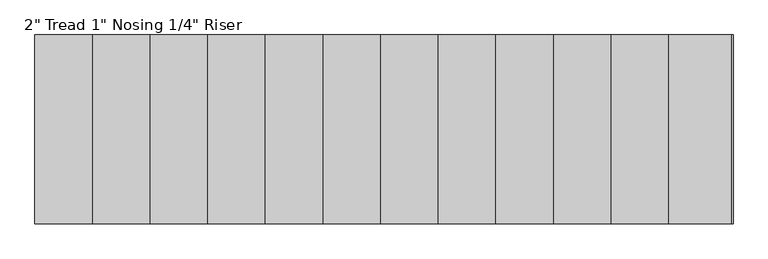
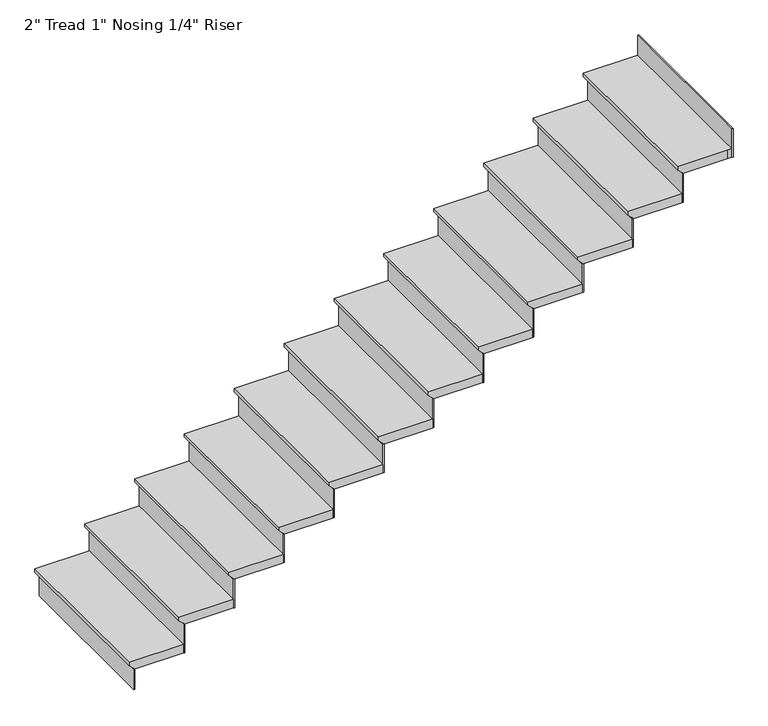
"""IFC4 building model written with IfcOpenShell, lengths in millimetres: stair flight geometry."""

from ifc_helpers import new_model, si_unit, origin, place, context, project, spatial, faceted_brep, source, transform, mapped, element, save


def stair_flight_2c1cbba1(model_context):
    return source(origin(), model_context, "Body", "Brep", [
        faceted_brep([(-3631.685793, -2823.2158798, 488.95), (-3631.685793, -2823.2158798, 508.0), (-3631.685793, -1908.8158798, 508.0), (-3631.685793, -1908.8158798, 488.95), (-3606.285793, -2823.2158798, 463.55), (-3606.285793, -1908.8158798, 463.55), (-3326.885793, -2823.2158798, 508.0), (-3326.885793, -1908.8158798, 508.0), (-3606.285793, -1908.8158798, 457.2), (-3326.885793, -1908.8158798, 457.2), (-3326.885793, -2823.2158798, 457.2), (-3606.285793, -2823.2158798, 457.2)], [[[0, 1, 2, 3]], [[4, 0, 3, 5]], [[2, 1, 6, 7]], [[8, 9, 10, 11]], [[2, 7, 9, 8, 5, 3]], [[8, 11, 4, 5]], [[6, 1, 0, 4, 11, 10]], [[7, 6, 10, 9]]]),
        faceted_brep([(-3606.285793, -2823.2158798, 457.2), (-3606.285793, -2823.2158798, 338.6666667), (-3599.935793, -2823.2158798, 338.6666667), (-3599.935793, -2823.2158798, 457.2), (-3606.285793, -1908.8158798, 457.2), (-3599.935793, -1908.8158798, 457.2), (-3599.935793, -1908.8158798, 338.6666667), (-3606.285793, -1908.8158798, 338.6666667)], [[[0, 1, 2, 3]], [[4, 5, 6, 7]], [[1, 0, 4, 7]], [[2, 1, 7, 6]], [[3, 2, 6, 5]], [[0, 3, 5, 4]]]),
        faceted_brep([(-3326.885793, -2823.2158798, 626.5333333), (-3326.885793, -2823.2158798, 457.2), (-3320.535793, -2823.2158798, 457.2), (-3320.535793, -2823.2158798, 626.5333333), (-3326.885793, -1908.8158798, 626.5333333), (-3320.535793, -1908.8158798, 626.5333333), (-3320.535793, -1908.8158798, 457.2), (-3326.885793, -1908.8158798, 457.2)], [[[0, 1, 2, 3]], [[4, 5, 6, 7]], [[1, 0, 4, 7]], [[2, 1, 7, 6]], [[3, 2, 6, 5]], [[0, 3, 5, 4]]]),
        faceted_brep([(-3352.285793, -1908.8158798, 677.3333333), (-3352.285793, -2823.2158798, 677.3333333), (-3047.485793, -2823.2158798, 677.3333333), (-3047.485793, -1908.8158798, 677.3333333), (-3326.885793, -1908.8158798, 626.5333333), (-3047.485793, -1908.8158798, 626.5333333), (-3047.485793, -2823.2158798, 626.5333333), (-3326.885793, -2823.2158798, 626.5333333), (-3326.885793, -1908.8158798, 632.8833333), (-3352.285793, -1908.8158798, 658.2833333), (-3326.885793, -2823.2158798, 632.8833333), (-3352.285793, -2823.2158798, 658.2833333)], [[[0, 1, 2, 3]], [[4, 5, 6, 7]], [[0, 3, 5, 4, 8, 9]], [[4, 7, 10, 8]], [[2, 1, 11, 10, 7, 6]], [[3, 2, 6, 5]], [[11, 1, 0, 9]], [[10, 11, 9, 8]]]),
        faceted_brep([(-3047.485793, -2823.2158798, 795.8666667), (-3047.485793, -2823.2158798, 626.5333333), (-3041.135793, -2823.2158798, 626.5333333), (-3041.135793, -2823.2158798, 795.8666667), (-3047.485793, -1908.8158798, 795.8666667), (-3041.135793, -1908.8158798, 795.8666667), (-3041.135793, -1908.8158798, 626.5333333), (-3047.485793, -1908.8158798, 626.5333333)], [[[0, 1, 2, 3]], [[4, 5, 6, 7]], [[1, 0, 4, 7]], [[2, 1, 7, 6]], [[3, 2, 6, 5]], [[0, 3, 5, 4]]]),
        faceted_brep([(-3072.885793, -1908.8158798, 846.6666667), (-3072.885793, -2823.2158798, 846.6666667), (-2768.085793, -2823.2158798, 846.6666667), (-2768.085793, -1908.8158798, 846.6666667), (-3047.485793, -1908.8158798, 795.8666667), (-2768.085793, -1908.8158798, 795.8666667), (-2768.085793, -2823.2158798, 795.8666667), (-3047.485793, -2823.2158798, 795.8666667), (-3047.485793, -1908.8158798, 802.2166667), (-3072.885793, -1908.8158798, 827.6166667), (-3047.485793, -2823.2158798, 802.2166667), (-3072.885793, -2823.2158798, 827.6166667)], [[[0, 1, 2, 3]], [[4, 5, 6, 7]], [[0, 3, 5, 4, 8, 9]], [[4, 7, 10, 8]], [[2, 1, 11, 10, 7, 6]], [[3, 2, 6, 5]], [[11, 1, 0, 9]], [[10, 11, 9, 8]]]),
        faceted_brep([(-2768.085793, -2823.2158798, 965.2), (-2768.085793, -2823.2158798, 795.8666667), (-2761.735793, -2823.2158798, 795.8666667), (-2761.735793, -2823.2158798, 965.2), (-2768.085793, -1908.8158798, 965.2), (-2761.735793, -1908.8158798, 965.2), (-2761.735793, -1908.8158798, 795.8666667), (-2768.085793, -1908.8158798, 795.8666667)], [[[0, 1, 2, 3]], [[4, 5, 6, 7]], [[1, 0, 4, 7]], [[2, 1, 7, 6]], [[3, 2, 6, 5]], [[0, 3, 5, 4]]]),
        faceted_brep([(-2793.485793, -1908.8158798, 1016.0), (-2793.485793, -2823.2158798, 1016.0), (-2488.685793, -2823.2158798, 1016.0), (-2488.685793, -1908.8158798, 1016.0), (-2768.085793, -1908.8158798, 965.2), (-2488.685793, -1908.8158798, 965.2), (-2488.685793, -2823.2158798, 965.2), (-2768.085793, -2823.2158798, 965.2), (-2768.085793, -1908.8158798, 971.55), (-2793.485793, -1908.8158798, 996.95), (-2768.085793, -2823.2158798, 971.55), (-2793.485793, -2823.2158798, 996.95)], [[[0, 1, 2, 3]], [[4, 5, 6, 7]], [[0, 3, 5, 4, 8, 9]], [[4, 7, 10, 8]], [[2, 1, 11, 10, 7, 6]], [[3, 2, 6, 5]], [[11, 1, 0, 9]], [[10, 11, 9, 8]]]),
        faceted_brep([(-2488.685793, -2823.2158798, 1134.5333333), (-2488.685793, -2823.2158798, 965.2), (-2482.335793, -2823.2158798, 965.2), (-2482.335793, -2823.2158798, 1134.5333333), (-2488.685793, -1908.8158798, 1134.5333333), (-2482.335793, -1908.8158798, 1134.5333333), (-2482.335793, -1908.8158798, 965.2), (-2488.685793, -1908.8158798, 965.2)], [[[0, 1, 2, 3]], [[4, 5, 6, 7]], [[1, 0, 4, 7]], [[2, 1, 7, 6]], [[3, 2, 6, 5]], [[0, 3, 5, 4]]]),
        faceted_brep([(-2514.085793, -1908.8158798, 1185.3333333), (-2514.085793, -2823.2158798, 1185.3333333), (-2209.285793, -2823.2158798, 1185.3333333), (-2209.285793, -1908.8158798, 1185.3333333), (-2488.685793, -1908.8158798, 1134.5333333), (-2209.285793, -1908.8158798, 1134.5333333), (-2209.285793, -2823.2158798, 1134.5333333), (-2488.685793, -2823.2158798, 1134.5333333), (-2488.685793, -1908.8158798, 1140.8833333), (-2514.085793, -1908.8158798, 1166.2833333), (-2488.685793, -2823.2158798, 1140.8833333), (-2514.085793, -2823.2158798, 1166.2833333)], [[[0, 1, 2, 3]], [[4, 5, 6, 7]], [[0, 3, 5, 4, 8, 9]], [[4, 7, 10, 8]], [[2, 1, 11, 10, 7, 6]], [[3, 2, 6, 5]], [[11, 1, 0, 9]], [[10, 11, 9, 8]]]),
        faceted_brep([(-2209.285793, -2823.2158798, 1303.8666667), (-2209.285793, -2823.2158798, 1134.5333333), (-2202.935793, -2823.2158798, 1134.5333333), (-2202.935793, -2823.2158798, 1303.8666667), (-2209.285793, -1908.8158798, 1303.8666667), (-2202.935793, -1908.8158798, 1303.8666667), (-2202.935793, -1908.8158798, 1134.5333333), (-2209.285793, -1908.8158798, 1134.5333333)], [[[0, 1, 2, 3]], [[4, 5, 6, 7]], [[1, 0, 4, 7]], [[2, 1, 7, 6]], [[3, 2, 6, 5]], [[0, 3, 5, 4]]]),
        faceted_brep([(-2234.685793, -1908.8158798, 1354.6666667), (-2234.685793, -2823.2158798, 1354.6666667), (-1929.885793, -2823.2158798, 1354.6666667), (-1929.885793, -1908.8158798, 1354.6666667), (-2209.285793, -1908.8158798, 1303.8666667), (-1929.885793, -1908.8158798, 1303.8666667), (-1929.885793, -2823.2158798, 1303.8666667), (-2209.285793, -2823.2158798, 1303.8666667), (-2209.285793, -1908.8158798, 1310.2166667), (-2234.685793, -1908.8158798, 1335.6166667), (-2209.285793, -2823.2158798, 1310.2166667), (-2234.685793, -2823.2158798, 1335.6166667)], [[[0, 1, 2, 3]], [[4, 5, 6, 7]], [[0, 3, 5, 4, 8, 9]], [[4, 7, 10, 8]], [[2, 1, 11, 10, 7, 6]], [[3, 2, 6, 5]], [[11, 1, 0, 9]], [[10, 11, 9, 8]]]),
        faceted_brep([(-1929.885793, -2823.2158798, 1473.2), (-1929.885793, -2823.2158798, 1303.8666667), (-1923.535793, -2823.2158798, 1303.8666667), (-1923.535793, -2823.2158798, 1473.2), (-1929.885793, -1908.8158798, 1473.2), (-1923.535793, -1908.8158798, 1473.2), (-1923.535793, -1908.8158798, 1303.8666667), (-1929.885793, -1908.8158798, 1303.8666667)], [[[0, 1, 2, 3]], [[4, 5, 6, 7]], [[1, 0, 4, 7]], [[2, 1, 7, 6]], [[3, 2, 6, 5]], [[0, 3, 5, 4]]]),
        faceted_brep([(-1955.285793, -1908.8158798, 1524.0), (-1955.285793, -2823.2158798, 1524.0), (-1650.485793, -2823.2158798, 1524.0), (-1650.485793, -1908.8158798, 1524.0), (-1929.885793, -1908.8158798, 1473.2), (-1650.485793, -1908.8158798, 1473.2), (-1650.485793, -2823.2158798, 1473.2), (-1929.885793, -2823.2158798, 1473.2), (-1929.885793, -1908.8158798, 1479.55), (-1955.285793, -1908.8158798, 1504.95), (-1929.885793, -2823.2158798, 1479.55), (-1955.285793, -2823.2158798, 1504.95)], [[[0, 1, 2, 3]], [[4, 5, 6, 7]], [[0, 3, 5, 4, 8, 9]], [[4, 7, 10, 8]], [[2, 1, 11, 10, 7, 6]], [[3, 2, 6, 5]], [[11, 1, 0, 9]], [[10, 11, 9, 8]]]),
        faceted_brep([(-1650.485793, -2823.2158798, 1642.5333333), (-1650.485793, -2823.2158798, 1473.2), (-1644.135793, -2823.2158798, 1473.2), (-1644.135793, -2823.2158798, 1642.5333333), (-1650.485793, -1908.8158798, 1642.5333333), (-1644.135793, -1908.8158798, 1642.5333333), (-1644.135793, -1908.8158798, 1473.2), (-1650.485793, -1908.8158798, 1473.2)], [[[0, 1, 2, 3]], [[4, 5, 6, 7]], [[1, 0, 4, 7]], [[2, 1, 7, 6]], [[3, 2, 6, 5]], [[0, 3, 5, 4]]]),
        faceted_brep([(-1675.885793, -1908.8158798, 1693.3333333), (-1675.885793, -2823.2158798, 1693.3333333), (-1371.085793, -2823.2158798, 1693.3333333), (-1371.085793, -1908.8158798, 1693.3333333), (-1650.485793, -1908.8158798, 1642.5333333), (-1371.085793, -1908.8158798, 1642.5333333), (-1371.085793, -2823.2158798, 1642.5333333), (-1650.485793, -2823.2158798, 1642.5333333), (-1650.485793, -1908.8158798, 1648.8833333), (-1675.885793, -1908.8158798, 1674.2833333), (-1650.485793, -2823.2158798, 1648.8833333), (-1675.885793, -2823.2158798, 1674.2833333)], [[[0, 1, 2, 3]], [[4, 5, 6, 7]], [[0, 3, 5, 4, 8, 9]], [[4, 7, 10, 8]], [[2, 1, 11, 10, 7, 6]], [[3, 2, 6, 5]], [[11, 1, 0, 9]], [[10, 11, 9, 8]]]),
        faceted_brep([(-1371.085793, -2823.2158798, 1811.8666667), (-1371.085793, -2823.2158798, 1642.5333333), (-1364.735793, -2823.2158798, 1642.5333333), (-1364.735793, -2823.2158798, 1811.8666667), (-1371.085793, -1908.8158798, 1811.8666667), (-1364.735793, -1908.8158798, 1811.8666667), (-1364.735793, -1908.8158798, 1642.5333333), (-1371.085793, -1908.8158798, 1642.5333333)], [[[0, 1, 2, 3]], [[4, 5, 6, 7]], [[1, 0, 4, 7]], [[2, 1, 7, 6]], [[3, 2, 6, 5]], [[0, 3, 5, 4]]]),
        faceted_brep([(-1396.485793, -1908.8158798, 1862.6666667), (-1396.485793, -2823.2158798, 1862.6666667), (-1091.685793, -2823.2158798, 1862.6666667), (-1091.685793, -1908.8158798, 1862.6666667), (-1371.085793, -1908.8158798, 1811.8666667), (-1091.685793, -1908.8158798, 1811.8666667), (-1091.685793, -2823.2158798, 1811.8666667), (-1371.085793, -2823.2158798, 1811.8666667), (-1371.085793, -1908.8158798, 1818.2166667), (-1396.485793, -1908.8158798, 1843.6166667), (-1371.085793, -2823.2158798, 1818.2166667), (-1396.485793, -2823.2158798, 1843.6166667)], [[[0, 1, 2, 3]], [[4, 5, 6, 7]], [[0, 3, 5, 4, 8, 9]], [[4, 7, 10, 8]], [[2, 1, 11, 10, 7, 6]], [[3, 2, 6, 5]], [[11, 1, 0, 9]], [[10, 11, 9, 8]]]),
        faceted_brep([(-1091.685793, -2823.2158798, 1981.2), (-1091.685793, -2823.2158798, 1811.8666667), (-1085.335793, -2823.2158798, 1811.8666667), (-1085.335793, -2823.2158798, 1981.2), (-1091.685793, -1908.8158798, 1981.2), (-1085.335793, -1908.8158798, 1981.2), (-1085.335793, -1908.8158798, 1811.8666667), (-1091.685793, -1908.8158798, 1811.8666667)], [[[0, 1, 2, 3]], [[4, 5, 6, 7]], [[1, 0, 4, 7]], [[2, 1, 7, 6]], [[3, 2, 6, 5]], [[0, 3, 5, 4]]]),
        faceted_brep([(-1117.085793, -1908.8158798, 2032.0), (-1117.085793, -2823.2158798, 2032.0), (-812.285793, -2823.2158798, 2032.0), (-812.285793, -1908.8158798, 2032.0), (-1091.685793, -1908.8158798, 1981.2), (-812.285793, -1908.8158798, 1981.2), (-812.285793, -2823.2158798, 1981.2), (-1091.685793, -2823.2158798, 1981.2), (-1091.685793, -1908.8158798, 1987.55), (-1117.085793, -1908.8158798, 2012.95), (-1091.685793, -2823.2158798, 1987.55), (-1117.085793, -2823.2158798, 2012.95)], [[[0, 1, 2, 3]], [[4, 5, 6, 7]], [[0, 3, 5, 4, 8, 9]], [[4, 7, 10, 8]], [[2, 1, 11, 10, 7, 6]], [[3, 2, 6, 5]], [[11, 1, 0, 9]], [[10, 11, 9, 8]]]),
        faceted_brep([(-812.285793, -2823.2158798, 2150.5333333), (-812.285793, -2823.2158798, 1981.2), (-805.935793, -2823.2158798, 1981.2), (-805.935793, -2823.2158798, 2150.5333333), (-812.285793, -1908.8158798, 2150.5333333), (-805.935793, -1908.8158798, 2150.5333333), (-805.935793, -1908.8158798, 1981.2), (-812.285793, -1908.8158798, 1981.2)], [[[0, 1, 2, 3]], [[4, 5, 6, 7]], [[1, 0, 4, 7]], [[2, 1, 7, 6]], [[3, 2, 6, 5]], [[0, 3, 5, 4]]]),
        faceted_brep([(-837.685793, -1908.8158798, 2201.3333333), (-837.685793, -2823.2158798, 2201.3333333), (-532.885793, -2823.2158798, 2201.3333333), (-532.885793, -1908.8158798, 2201.3333333), (-812.285793, -1908.8158798, 2150.5333333), (-532.885793, -1908.8158798, 2150.5333333), (-532.885793, -2823.2158798, 2150.5333333), (-812.285793, -2823.2158798, 2150.5333333), (-812.285793, -1908.8158798, 2156.8833333), (-837.685793, -1908.8158798, 2182.2833333), (-812.285793, -2823.2158798, 2156.8833333), (-837.685793, -2823.2158798, 2182.2833333)], [[[0, 1, 2, 3]], [[4, 5, 6, 7]], [[0, 3, 5, 4, 8, 9]], [[4, 7, 10, 8]], [[2, 1, 11, 10, 7, 6]], [[3, 2, 6, 5]], [[11, 1, 0, 9]], [[10, 11, 9, 8]]]),
        faceted_brep([(-532.885793, -2823.2158798, 2319.8666667), (-532.885793, -2823.2158798, 2150.5333333), (-526.535793, -2823.2158798, 2150.5333333), (-526.535793, -2823.2158798, 2319.8666667), (-532.885793, -1908.8158798, 2319.8666667), (-526.535793, -1908.8158798, 2319.8666667), (-526.535793, -1908.8158798, 2150.5333333), (-532.885793, -1908.8158798, 2150.5333333)], [[[0, 1, 2, 3]], [[4, 5, 6, 7]], [[1, 0, 4, 7]], [[2, 1, 7, 6]], [[3, 2, 6, 5]], [[0, 3, 5, 4]]]),
        faceted_brep([(-253.485793, -2823.2158798, 2489.2), (-253.485793, -2823.2158798, 2319.8666667), (-247.135793, -2823.2158798, 2319.8666667), (-247.135793, -2823.2158798, 2489.2), (-253.485793, -1908.8158798, 2489.2), (-247.135793, -1908.8158798, 2489.2), (-247.135793, -1908.8158798, 2319.8666667), (-253.485793, -1908.8158798, 2319.8666667)], [[[0, 1, 2, 3]], [[4, 5, 6, 7]], [[1, 0, 4, 7]], [[2, 1, 7, 6]], [[3, 2, 6, 5]], [[0, 3, 5, 4]]]),
        faceted_brep([(-253.485793, -1908.8158798, 2370.6666667), (-278.885793, -1908.8158798, 2370.6666667), (-558.285793, -1908.8158798, 2370.6666667), (-558.285793, -2823.2158798, 2370.6666667), (-278.885793, -2823.2158798, 2370.6666667), (-253.485793, -2823.2158798, 2370.6666667), (-278.885793, -1908.8158798, 2319.8666667), (-253.485793, -1908.8158798, 2319.8666667), (-253.485793, -2823.2158798, 2319.8666667), (-278.885793, -2823.2158798, 2319.8666667), (-532.885793, -2823.2158798, 2319.8666667), (-532.885793, -1908.8158798, 2319.8666667), (-532.885793, -1908.8158798, 2326.2166667), (-558.285793, -1908.8158798, 2351.6166667), (-532.885793, -2823.2158798, 2326.2166667), (-558.285793, -2823.2158798, 2351.6166667)], [[[0, 1, 2, 3, 4, 5]], [[6, 7, 8, 9, 10, 11]], [[1, 0, 7, 6]], [[2, 1, 6, 11, 12, 13]], [[11, 10, 14, 12]], [[4, 3, 15, 14, 10, 9]], [[5, 4, 9, 8]], [[0, 5, 8, 7]], [[15, 3, 2, 13]], [[14, 15, 13, 12]]]),
    ])


if __name__ == "__main__":
    model = new_model("IFC4")
    model_context = context("Model", 3, world=origin())
    ifc_project = project(units=[si_unit("LENGTHUNIT", "METRE", prefix="MILLI")], contexts=[model_context])
    site = spatial("IfcSite", under=ifc_project)
    building = spatial("IfcBuilding", under=site)
    placement = place(None, origin())
    stair_flight_shape = stair_flight_2c1cbba1(model_context)
    element("IfcStairFlight", 1, ObjectType="2\" Tread 1\" Nosing 1/4\" Riser", at=placement, inside=building, context=model_context, shape_type="MappedRepresentation", body=[
        mapped(stair_flight_shape, transform((0.0, 0.0, 0.0), x_axis=(1.0, 0.0, 0.0), y_axis=(0.0, 1.0, 0.0), z_axis=(0.0, 0.0, 1.0))),
    ])
    save(model, "model.ifc")
